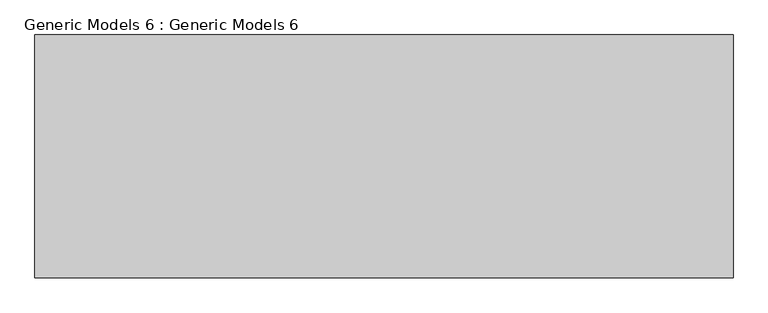
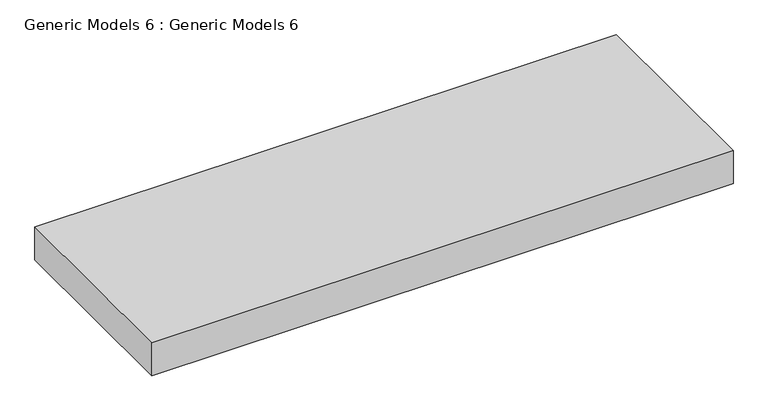
"""IFC4 building model written with IfcOpenShell, lengths in millimetres: proxy geometry, Generic Models 6 : Generic Models 6."""

from ifc_helpers import new_model, si_unit, frame, origin, place, context, project, spatial, polyline, outline, extrude, source, transform, mapped, element, save


def generic_models_6_generic_models_6_1132ce1b(model_context):
    return source(origin(), model_context, "Body", "SweptSolid", [
        extrude(outline(polyline([(-14897.4864432, 3355.3054373), (-14897.4864432, 4690.9207268), (-11060.6574599, 4690.9207268), (-11060.6574599, 3355.3054373), (-14897.4864432, 3355.3054373)])), frame((0.0, 0.0, 2408.3377855), z_axis=(0.0, 0.0, 1.0), x_axis=(1.0, 0.0, 0.0)), (0.0, 0.0, 1.0), 228.6),
    ])


if __name__ == "__main__":
    model = new_model("IFC4")
    model_context = context("Model", 3, world=origin())
    ifc_project = project(units=[si_unit("LENGTHUNIT", "METRE", prefix="MILLI")], contexts=[model_context])
    site = spatial("IfcSite", under=ifc_project)
    building = spatial("IfcBuilding", under=site)
    placement = place(None, origin())
    generic_models_6_generic_models_6_shape = generic_models_6_generic_models_6_1132ce1b(model_context)
    element("IfcBuildingElementProxy", 1, Name="Generic Models 6 : Generic Models 6", ObjectType="Generic Models 6 : Generic Models 6", at=placement, inside=building, context=model_context, shape_type="MappedRepresentation", body=[
        mapped(generic_models_6_generic_models_6_shape, transform((0.0, 0.0, 0.0), x_axis=(1.0, 0.0, 0.0), y_axis=(0.0, 1.0, 0.0), z_axis=(0.0, 0.0, 1.0))),
    ])
    save(model, "model.ifc")
